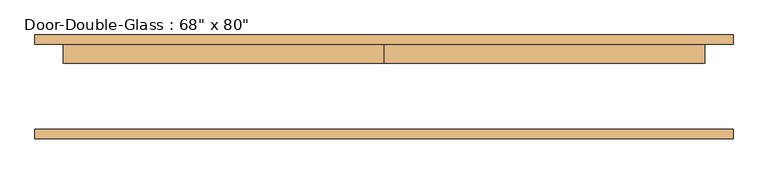
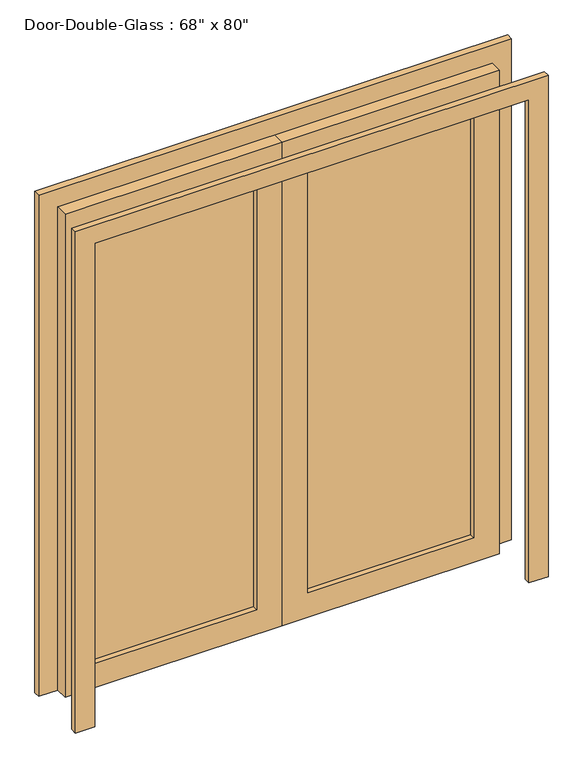
"""IFC4 building model written with IfcOpenShell, lengths in millimetres: door geometry."""

from ifc_helpers import new_model, si_unit, frame, origin, place, context, project, spatial, polyline, outline, extrude, source, transform, mapped, element, save


def door_bbcd5f29(model_context):
    return source(origin(), model_context, "Body", "SweptSolid", [
        extrude(outline(polyline([(2032.0, 863.6), (2032.0, 0.0), (0.0, 0.0), (0.0, 863.6), (2032.0, 863.6)]), holes=[polyline([(1930.4, 762.0), (101.6, 762.0), (101.6, 101.6), (1930.4, 101.6), (1930.4, 762.0)])]), frame((0.0, 65.88125, 0.0), z_axis=(0.0, 1.0, 0.0), x_axis=(0.0, 0.0, 1.0)), (0.0, 0.0, 1.0), 50.8),
        extrude(outline(polyline([(2032.0, -863.6), (0.0, -863.6), (0.0, 0.0), (2032.0, 0.0), (2032.0, -863.6)]), holes=[polyline([(1930.4, -762.0), (1930.4, -101.6), (101.6, -101.6), (101.6, -762.0), (1930.4, -762.0)])]), frame((0.0, 65.88125, 0.0), z_axis=(0.0, 1.0, 0.0), x_axis=(0.0, 0.0, 1.0)), (0.0, 0.0, 1.0), 50.8),
        extrude(outline(polyline([(-762.0, 94.45625), (-101.6, 94.45625), (-101.6, 88.10625), (-762.0, 88.10625), (-762.0, 94.45625)])), frame((0.0, 0.0, 101.6), z_axis=(0.0, 0.0, 1.0), x_axis=(1.0, 0.0, 0.0)), (0.0, 0.0, 1.0), 1828.8),
        extrude(outline(polyline([(101.6, 94.45625), (762.0, 94.45625), (762.0, 88.10625), (101.6, 88.10625), (101.6, 94.45625)])), frame((0.0, 0.0, 101.6), z_axis=(0.0, 0.0, 1.0), x_axis=(1.0, 0.0, 0.0)), (0.0, 0.0, 1.0), 1828.8),
        extrude(outline(polyline([(0.0, 939.8), (2108.2, 939.8), (2108.2, -939.8), (0.0, -939.8), (0.0, -863.6), (2032.0, -863.6), (2032.0, 863.6), (0.0, 863.6), (0.0, 939.8)])), frame((0.0, -137.31875, 0.0), z_axis=(0.0, 1.0, 0.0), x_axis=(0.0, 0.0, 1.0)), (0.0, 0.0, 1.0), 25.4),
        extrude(outline(polyline([(0.0, 939.8), (2108.2, 939.8), (2108.2, -939.8), (0.0, -939.8), (0.0, -863.6), (2032.0, -863.6), (2032.0, 863.6), (0.0, 863.6), (0.0, 939.8)])), frame((0.0, 116.68125, 0.0), z_axis=(0.0, 1.0, 0.0), x_axis=(0.0, 0.0, 1.0)), (0.0, 0.0, 1.0), 25.4),
    ])


if __name__ == "__main__":
    model = new_model("IFC4")
    model_context = context("Model", 3, world=origin())
    ifc_project = project(units=[si_unit("LENGTHUNIT", "METRE", prefix="MILLI")], contexts=[model_context])
    site = spatial("IfcSite", under=ifc_project)
    building = spatial("IfcBuilding", under=site)
    placement = place(None, origin())
    door_shape = door_bbcd5f29(model_context)
    element("IfcDoor", 1, ObjectType="Door-Double-Glass : 68\" x 80\"", at=placement, inside=building, context=model_context, shape_type="MappedRepresentation", body=[
        mapped(door_shape, transform((0.0, 0.0, 0.0), x_axis=(1.0, 0.0, 0.0), y_axis=(0.0, 1.0, 0.0), z_axis=(0.0, 0.0, 1.0))),
    ])
    save(model, "model.ifc")

# Revit data of these elements
# Type "Door-Double-Glass : 68\" x 80\""
#   Type Mark = "46"
#   Construction Type Id = "opn-d45"
#   Assembly Code = "C1020"
#   Analytic Construction = "Wood frame, double glass door "
#   W = 2' - 10"
#   Thickness = 0' - 2"
#   Thermal Resistance (R) = 0.31964 (m²·K)/W
#   Swing Angle [instance default] = 90.00°
#   Heat Transfer Coefficient (U) = 3.12872 W/(m²·K)
#   Height = 6' - 8"
#   Bottom Rail = 0' - 4"
#   Top Rail = 0' - 4"
#   Stiles = 0' - 4"
#   Trim Projection = 0' - 1"
#   Trim Width = 0' - 3"
#   Width = 5' - 8"
#   Define Thermal Properties by = 1
#   Glazing = Glass
#   Panel Material = Wood - Birch - Solid Stained Light Low Gloss
#   Trim Material = Paint - Sienna
#   Visual Light Transmittance = 0
#   Solar Heat Gain Coefficient = 0
#   Function = (empty or 0)
#   Wall Closure = (empty or 0)
# Element 1 (IfcDoor, "Door-Double-Glass : 68\" x 80\"")
#   Materials on its faces: "Wood - Birch - Solid Stained Light Low Gloss", "Paint - Sienna", "Glass"
# Materials
#   "Glass": class "Glass", colour RGB 0 128 192, transparency 0.9, Description = "Soda Lime Glass", Cost = 0
#   "Wood - Birch - Solid Stained Light Low Gloss": class "Wood", colour RGB 210 159 95, transparency 0, Cost = 0
#   "Paint - Sienna": colour RGB 118 70 51, transparency 0, Cost = 0
